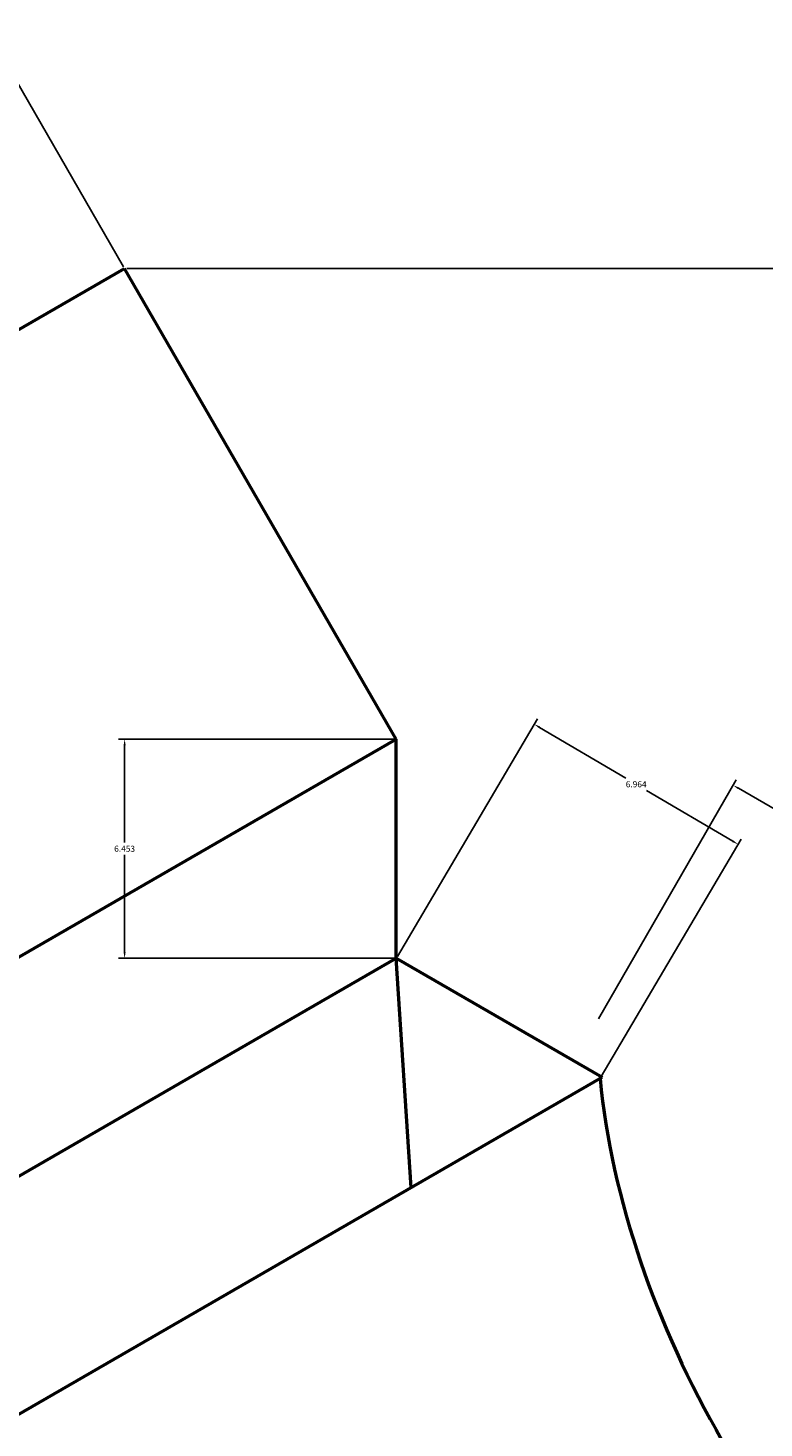
# Model space of a CAD drawing. Units: millimetres. Extents: x 2919 to 3075, y 2801 to 2951.
# Tile 9 of 14: x 2984 to 3006, y 2910 to 2951. Entities that reach past the tile are written whole.
import ezdxf

# ---------------------------------------------------------------- set-up
doc = ezdxf.new("R2010")
doc.units = ezdxf.units.MM
doc.layers.add('M-DIMS', color=2, linetype='Continuous', lineweight=18)
doc.layers.add('M-OUTL', color=7, linetype='Continuous', lineweight=50)
doc.styles.get("Standard").update_dxf_attribs({"font": 'arial.ttf'})
doc.dimstyles.get("Standard").update_dxf_attribs({"dimtxt": 0.18, "dimasz": 0.18, "dimexe": 0.18, "dimexo": 0.0625, "dimgap": 0.09, "dimtad": 0, "dimtih": 1, "dimtoh": 1, "dimdec": 4, "dimzin": 0, "dimdsep": 46, "dimtxsty": 'Standard', "dimcen": 0.09, "dimadec": 0, "dimazin": 0, "dimtfac": 1, "dimtdec": 4, "dimtofl": 0, "dimtmove": 0, "dimatfit": 3, "dimfxl": 1, "dimtolj": 1, "dimtzin": 0, "dimarcsym": 0})

# ---------------------------------------------------------------- blocks, each defined once
blk = doc.blocks.new('*D1')
at = {"layer": 'Defpoints', "color": 0, "transparency": 16777216}
for p in [(2987.323, 2944.203), (3074.337, 2944.203), (3010.912, 2808.893)]:
    blk.add_point(p, dxfattribs=at)
at = {"layer": 'M-DIMS', "color": 0, "lineweight": -2, "transparency": 16777216}
for p, q in [((2987.386, 2944.203), (3074.517, 2944.203)), ((3074.337, 2944.023), (3074.337, 2876.73)), ((3074.337, 2809.073), (3074.337, 2876.366)), ((3010.974, 2808.893), (3074.517, 2808.893))]:
    blk.add_line(p, q, dxfattribs=at)
at = {"layer": 'M-DIMS', "color": 0, "transparency": 16777216}
for points in [[(3074.307, 2944.023), (3074.367, 2944.023), (3074.337, 2944.203)], [(3074.307, 2809.073), (3074.367, 2809.073), (3074.337, 2808.893)]]:
    blk.add_solid(points, dxfattribs=at)
at = {"layer": 'M-DIMS', "color": 0, "transparency": 16777216, "insert": (3074.337, 2876.548), "char_height": 0.18, "attachment_point": 5}
blk.add_mtext('\\A1;135.3', dxfattribs=at)
blk = doc.blocks.new('*D16')
at = {"layer": 'Defpoints', "color": 0, "transparency": 16777216}
for p in [(2983.323, 2951.131), (2987.323, 2944.203), (2950.626, 2923.015)]:
    blk.add_point(p, dxfattribs=at)
at = {"layer": 'M-DIMS', "color": 0, "lineweight": -2, "transparency": 16777216}
for p, q in [((2987.292, 2944.257), (2983.233, 2951.287)), ((2983.167, 2951.041), (2965.29, 2940.719)), ((2946.782, 2930.034), (2964.659, 2940.355)), ((2950.595, 2923.07), (2946.536, 2930.1))]:
    blk.add_line(p, q, dxfattribs=at)
at = {"layer": 'M-DIMS', "color": 0, "transparency": 16777216}
for points in [[(2983.152, 2951.067), (2983.182, 2951.015), (2983.323, 2951.131)], [(2946.767, 2930.06), (2946.797, 2930.008), (2946.626, 2929.944)]]:
    blk.add_solid(points, dxfattribs=at)
at = {"layer": 'M-DIMS', "color": 0, "transparency": 16777216, "insert": (2964.975, 2940.537), "char_height": 0.18, "attachment_point": 5}
blk.add_mtext('\\A1;42.374', dxfattribs=at)
blk = doc.blocks.new('*D18')
at = {"layer": 'Defpoints', "color": 0, "transparency": 16777216}
for p in [(3001.241, 2922.061), (3030.348, 2914.493), (3026.348, 2907.565)]:
    blk.add_point(p, dxfattribs=at)
at = {"layer": 'M-DIMS', "color": 0, "lineweight": -2, "transparency": 16777216}
for p, q in [((3001.272, 2922.115), (3005.331, 2929.145)), ((3005.397, 2928.899), (3017.471, 2921.928)), ((3030.192, 2914.583), (3018.118, 2921.554)), ((3026.379, 2907.619), (3030.438, 2914.649))]:
    blk.add_line(p, q, dxfattribs=at)
at = {"layer": 'M-DIMS', "color": 0, "transparency": 16777216}
for points in [[(3005.412, 2928.925), (3005.382, 2928.873), (3005.241, 2928.989)], [(3030.207, 2914.609), (3030.177, 2914.557), (3030.348, 2914.493)]]:
    blk.add_solid(points, dxfattribs=at)
at = {"layer": 'M-DIMS', "color": 0, "transparency": 16777216, "insert": (3017.794, 2921.741), "char_height": 0.18, "attachment_point": 5}
blk.add_mtext('\\A1;%%c28.99', dxfattribs=at)
blk = doc.blocks.new('*D19')
at = {"layer": 'Defpoints', "color": 0, "transparency": 16777216}
for p in [(2987.323, 2930.346), (2995.323, 2930.346), (2995.323, 2923.893)]:
    blk.add_point(p, dxfattribs=at)
at = {"layer": 'M-DIMS', "color": 0, "lineweight": -2, "transparency": 16777216}
for p, q in [((2995.261, 2930.346), (2987.143, 2930.346)), ((2987.323, 2930.166), (2987.323, 2927.302)), ((2987.323, 2924.073), (2987.323, 2926.938)), ((2995.261, 2923.893), (2987.143, 2923.893))]:
    blk.add_line(p, q, dxfattribs=at)
at = {"layer": 'M-DIMS', "color": 0, "transparency": 16777216}
for points in [[(2987.293, 2930.166), (2987.353, 2930.166), (2987.323, 2930.346)], [(2987.293, 2924.073), (2987.353, 2924.073), (2987.323, 2923.893)]]:
    blk.add_solid(points, dxfattribs=at)
at = {"layer": 'M-DIMS', "color": 0, "transparency": 16777216, "insert": (2987.323, 2927.12), "char_height": 0.18, "attachment_point": 5}
blk.add_mtext('\\A1;6.453', dxfattribs=at)
blk = doc.blocks.new('*D24')
at = {"layer": 'Defpoints', "color": 0, "transparency": 16777216}
for p in [(3005.385, 2927.25), (2995.323, 2923.893), (3001.323, 2920.357)]:
    blk.add_point(p, dxfattribs=at)
at = {"layer": 'M-DIMS', "color": 0, "lineweight": -2, "transparency": 16777216}
for p, q in [((2995.355, 2923.947), (2999.476, 2930.941)), ((2999.54, 2930.694), (3002.076, 2929.199)), ((3005.23, 2927.341), (3002.694, 2928.836)), ((3001.355, 2920.411), (3005.476, 2927.405))]:
    blk.add_line(p, q, dxfattribs=at)
at = {"layer": 'M-DIMS', "color": 0, "transparency": 16777216}
for points in [[(2999.555, 2930.72), (2999.525, 2930.668), (2999.385, 2930.785)], [(3005.245, 2927.367), (3005.215, 2927.315), (3005.385, 2927.25)]]:
    blk.add_solid(points, dxfattribs=at)
at = {"layer": 'M-DIMS', "color": 0, "transparency": 16777216, "insert": (3002.385, 2929.018), "char_height": 0.18, "attachment_point": 5}
blk.add_mtext('\\A1;6.964', dxfattribs=at)

msp = doc.modelspace()

# ---------------------------------------------------------------- linework, layer by layer
at = {"layer": 'M-OUTL'}
for p, q in [((2995.3232, 2930.3462), (2987.3232, 2944.2026)), ((2995.3232, 2923.8932), (2995.3232, 2930.3462)), ((2960.6821, 2903.8932), (2995.3232, 2923.8932)), ((2995.7562, 2917.1432), (2995.3232, 2923.8932)), ((2995.3232, 2923.8932), (3001.3853, 2920.3932)), ((2966.7443, 2900.3932), (3001.3853, 2920.3932))]:
    msp.add_line(p, q, dxfattribs=at)
for points in [[(2928.6099, 2892.1931), (2950.6258, 2923.0154), (2987.3232, 2944.2026)], [(2941.6296, 2882.8932), (2961.6296, 2910.8932), (2995.3232, 2930.3462)], [(2941.6296, 2882.8932), (2961.6296, 2910.8932), (2995.3232, 2930.3462)]]:
    msp.add_lwpolyline(points, dxfattribs=at)
msp.add_ellipse((3013.7944, 2914.8129), major_axis=(8.8766, -15.3748), ratio=0.5773503, start_param=4.0414742, end_param=5.3833038, dxfattribs=at)

# ---------------------------------------------------------------- dimensions: what is measured, and where the dimension line sits
at = {"layer": 'M-DIMS'}
for base, p1, p2, angle, override, picture, middle in [((2983.3232, 2951.1308), (2950.6258, 2923.0154), (2987.3232, 2944.2026), 30, {"dimdec": 3, "dimlfac": 1, "dimrnd": 0, "dimzin": 0, "dimdsep": 46, "dimlunit": 2}, '*D16', (2964.9745, 2940.5372)), ((3074.3372, 2944.2026), (3010.9116, 2808.8932), (2987.3232, 2944.2026), 90, {"dimdec": 1, "dimlfac": 1, "dimrnd": 0, "dimzin": 0, "dimdsep": 46, "dimlunit": 2}, '*D1', (3074.3372, 2876.5479)), ((3005.3849, 2927.2496), (2995.3232, 2923.8932), (3001.3232, 2920.3574), 329.48858, {"dimdec": 3, "dimlfac": 1, "dimrnd": 0, "dimzin": 0, "dimdsep": 46, "dimlunit": 2}, '*D24', (3002.3849, 2929.0175)), ((2987.3232, 2930.3462), (2995.3232, 2923.8932), (2995.3232, 2930.3462), 90, {"dimdec": 3, "dimlfac": 1, "dimrnd": 0, "dimzin": 0, "dimdsep": 46, "dimlunit": 2}, '*D19', (2987.3232, 2927.1197))]:
    dim = msp.add_linear_dim(base=base, p1=p1, p2=p2, angle=angle, dimstyle='Standard', override=override, dxfattribs=at)
    dim.commit()
    dim.dimension.update_dxf_attribs({"geometry": picture, "text_midpoint": middle})
dim = msp.add_linear_dim(base=(3030.3479, 2914.4934), p1=(3001.241, 2922.0607), p2=(3026.3479, 2907.5652), angle=330, text='%%c<>', dimstyle='Standard', override={"dimdec": 2, "dimlfac": 1, "dimrnd": 0, "dimzin": 0, "dimdsep": 46, "dimlunit": 2}, dxfattribs=at)
dim.commit()
dim.dimension.update_dxf_attribs({"geometry": '*D18', "text_midpoint": (3017.7944, 2921.7411)})

doc.saveas('drawing.dxf')
